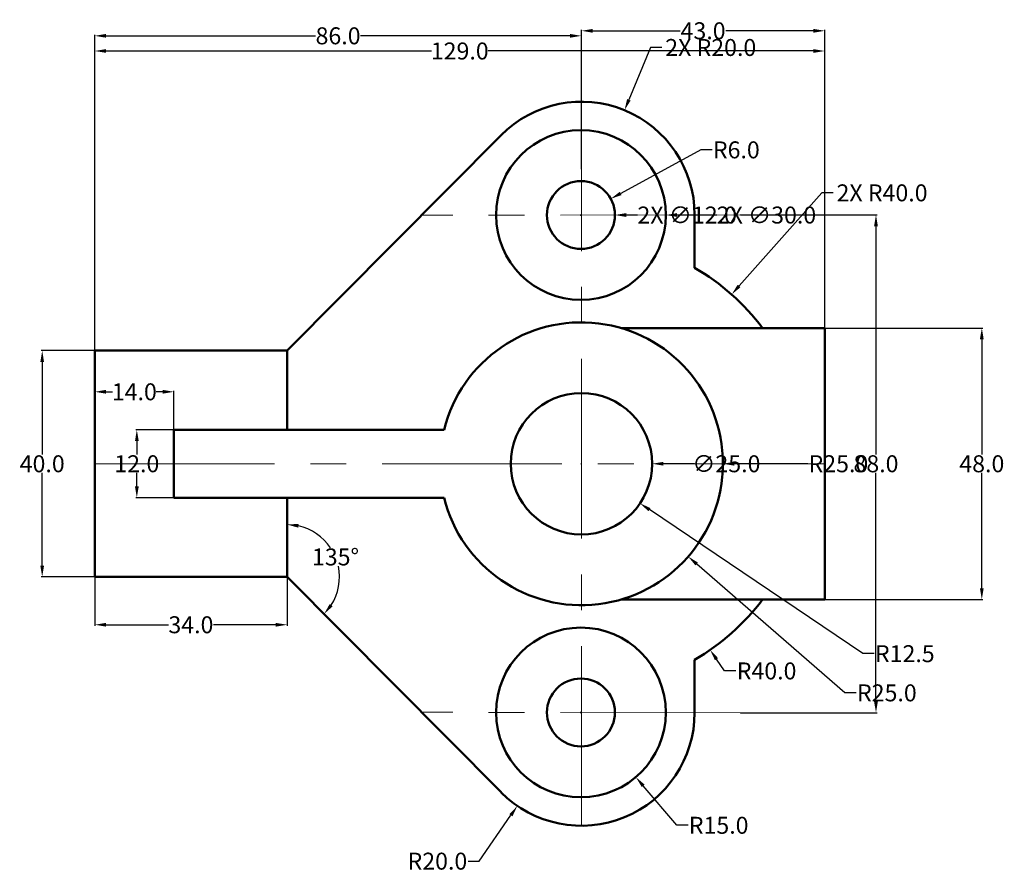
# Model space of a CAD drawing. Units: inches. Extents: x 158 to 332, y 82 to 233.
import ezdxf

# ---------------------------------------------------------------- set-up
doc = ezdxf.new("R2010")
doc.units = ezdxf.units.IN
doc.header["$MEASUREMENT"] = 0
doc.linetypes.add('CENTER', pattern=[50.8, 31.75, -6.35, 6.35, -6.35])
for name, color, linetype, lineweight in [('M-CNTR', 4, 'CENTER', 18), ('M-CONS', 8, 'Continuous', 13), ('M-DIMS', 2, 'Continuous', 25), ('M-OUTL', 7, 'Continuous', 50)]:
    doc.layers.add(name, color=color, linetype=linetype, lineweight=lineweight)
doc.styles.get("Standard").update_dxf_attribs({"font": 'arial.ttf'})
doc.dimstyles.get("Standard").update_dxf_attribs({"dimtxt": 3, "dimasz": 2, "dimexe": 0.18, "dimexo": 0.0625, "dimgap": 0.09, "dimtad": 0, "dimtih": 1, "dimtoh": 1, "dimdec": 1, "dimzin": 0, "dimdsep": 46, "dimtxsty": 'Standard', "dimcen": 0.09, "dimadec": 0, "dimazin": 0, "dimtfac": 1, "dimtdec": 1, "dimtofl": 0, "dimtmove": 0, "dimatfit": 3, "dimfxl": 1, "dimtolj": 1, "dimtzin": 0, "dimarcsym": 0})

# ---------------------------------------------------------------- blocks, each defined once
blk = doc.blocks.new('*D1')
at = {"layer": 'Defpoints', "color": 0, "transparency": 16777216}
for p in [(178.74, 160.59), (185.3, 160.59), (185.3, 148.59)]:
    blk.add_point(p, dxfattribs=at)
at = {"layer": 'M-DIMS', "color": 0, "lineweight": -2, "transparency": 16777216}
for p, q in [((185.24, 160.59), (178.56, 160.59)), ((178.74, 158.59), (178.74, 156.22)), ((178.74, 150.59), (178.74, 152.97)), ((185.24, 148.59), (178.56, 148.59))]:
    blk.add_line(p, q, dxfattribs=at)
at = {"layer": 'M-DIMS', "color": 0, "transparency": 16777216}
for points in [[(178.41, 158.59), (179.08, 158.59), (178.74, 160.59)], [(178.41, 150.59), (179.08, 150.59), (178.74, 148.59)]]:
    blk.add_solid(points, dxfattribs=at)
at = {"layer": 'M-DIMS', "color": 0, "transparency": 16777216, "insert": (178.74, 154.59), "char_height": 3, "attachment_point": 5}
blk.add_mtext('\\A1;12.0', dxfattribs=at)
blk = doc.blocks.new('*D2')
at = {"layer": 'Defpoints', "color": 0, "transparency": 16777216}
for p in [(171.3, 167.31), (185.3, 167.31), (185.3, 160.59)]:
    blk.add_point(p, dxfattribs=at)
at = {"layer": 'M-DIMS', "color": 0, "lineweight": -2, "transparency": 16777216}
for p, q in [((171.3, 167.38), (171.3, 167.49)), ((173.3, 167.31), (174.46, 167.31)), ((183.3, 167.31), (182.14, 167.31)), ((185.3, 160.66), (185.3, 167.49))]:
    blk.add_line(p, q, dxfattribs=at)
at = {"layer": 'M-DIMS', "color": 0, "transparency": 16777216}
for points in [[(173.3, 167.65), (173.3, 166.98), (171.3, 167.31)], [(183.3, 167.65), (183.3, 166.98), (185.3, 167.31)]]:
    blk.add_solid(points, dxfattribs=at)
at = {"layer": 'M-DIMS', "color": 0, "transparency": 16777216, "insert": (178.3, 167.31), "char_height": 3, "attachment_point": 5}
blk.add_mtext('\\A1;14.0', dxfattribs=at)
blk = doc.blocks.new('*D3')
at = {"layer": 'Defpoints', "color": 0, "transparency": 16777216}
for p in [(171.3, 134.59), (205.3, 134.59), (205.3, 126.13)]:
    blk.add_point(p, dxfattribs=at)
at = {"layer": 'M-DIMS', "color": 0, "lineweight": -2, "transparency": 16777216}
for p, q in [((171.3, 134.53), (171.3, 125.95)), ((205.3, 134.53), (205.3, 125.95)), ((173.3, 126.13), (184.32, 126.13)), ((203.3, 126.13), (192.28, 126.13))]:
    blk.add_line(p, q, dxfattribs=at)
at = {"layer": 'M-DIMS', "color": 0, "transparency": 16777216}
for points in [[(173.3, 126.46), (173.3, 125.8), (171.3, 126.13)], [(203.3, 126.46), (203.3, 125.8), (205.3, 126.13)]]:
    blk.add_solid(points, dxfattribs=at)
at = {"layer": 'M-DIMS', "color": 0, "transparency": 16777216, "insert": (188.3, 126.13), "char_height": 3, "attachment_point": 5}
blk.add_mtext('\\A1;34.0', dxfattribs=at)
blk = doc.blocks.new('*D4')
at = {"layer": 'Defpoints', "color": 0, "transparency": 16777216}
for p in [(162.02, 174.59), (171.3, 174.59), (171.3, 134.59)]:
    blk.add_point(p, dxfattribs=at)
at = {"layer": 'M-DIMS', "color": 0, "lineweight": -2, "transparency": 16777216}
for p, q in [((171.24, 174.59), (161.84, 174.59)), ((162.02, 172.59), (162.02, 156.22)), ((162.02, 136.59), (162.02, 152.97)), ((171.24, 134.59), (161.84, 134.59))]:
    blk.add_line(p, q, dxfattribs=at)
at = {"layer": 'M-DIMS', "color": 0, "transparency": 16777216}
for points in [[(161.69, 172.59), (162.35, 172.59), (162.02, 174.59)], [(161.69, 136.59), (162.35, 136.59), (162.02, 134.59)]]:
    blk.add_solid(points, dxfattribs=at)
at = {"layer": 'M-DIMS', "color": 0, "transparency": 16777216, "insert": (162.02, 154.59), "char_height": 3, "attachment_point": 5}
blk.add_mtext('\\A1;40.0', dxfattribs=at)
blk = doc.blocks.new('*D5')
at = {"layer": 'Defpoints', "color": 0, "transparency": 16777216}
for p in [(205.3, 148.59), (205.3, 134.59), (205.3, 134.59), (214.55, 134.57), (243.1, 96.51)]:
    blk.add_point(p, dxfattribs=at)
at = {"layer": 'M-DIMS', "color": 0, "lineweight": -2, "transparency": 16777216}
for start, end in [(33.8017, 77.592), (327.1935, 11.8638)]:
    blk.add_arc((205.3, 134.59), 9.25, start, end, dxfattribs=at)
at = {"layer": 'M-DIMS', "color": 0, "transparency": 16777216}
for points in [[(207.25, 143.3), (207.32, 143.96), (205.3, 143.85)], [(213.33, 129.37), (212.82, 129.79), (211.82, 128.03)]]:
    blk.add_solid(points, dxfattribs=at)
at = {"layer": 'M-DIMS', "color": 0, "transparency": 16777216, "insert": (213.85, 138.12), "char_height": 3, "attachment_point": 5}
blk.add_mtext('\\A1;135°', dxfattribs=at)
blk = doc.blocks.new('*D6')
at = {"layer": 'Defpoints', "color": 0, "transparency": 16777216}
for p in [(257.3, 110.59), (245.98, 94.11)]:
    blk.add_point(p, dxfattribs=at)
at = {"layer": 'M-DIMS', "color": 0, "lineweight": -2, "transparency": 16777216}
for p, q in [((257.21, 110.59), (257.39, 110.59)), ((257.3, 110.5), (257.3, 110.68)), ((239.26, 84.34), (244.84, 92.46)), ((237.26, 84.34), (239.26, 84.34))]:
    blk.add_line(p, q, dxfattribs=at)
at = {"layer": 'M-DIMS', "color": 0, "transparency": 16777216}
blk.add_solid([(244.57, 92.65), (245.12, 92.27), (245.98, 94.11)], dxfattribs=at)
at = {"layer": 'M-DIMS', "color": 0, "transparency": 16777216, "insert": (231.85, 84.34), "char_height": 3, "attachment_point": 5}
blk.add_mtext('\\A1;R20.0', dxfattribs=at)
blk = doc.blocks.new('*D7')
at = {"layer": 'Defpoints', "color": 0, "transparency": 16777216}
for p in [(257.21, 110.63), (266.92, 99.19)]:
    blk.add_point(p, dxfattribs=at)
at = {"layer": 'M-DIMS', "color": 0, "lineweight": -2, "transparency": 16777216}
for p, q in [((257.12, 110.63), (257.3, 110.63)), ((257.21, 110.54), (257.21, 110.72)), ((274.14, 90.68), (268.21, 97.67)), ((276.14, 90.68), (274.14, 90.68))]:
    blk.add_line(p, q, dxfattribs=at)
at = {"layer": 'M-DIMS', "color": 0, "transparency": 16777216}
blk.add_solid([(268.46, 97.88), (267.96, 97.45), (266.92, 99.19)], dxfattribs=at)
at = {"layer": 'M-DIMS', "color": 0, "transparency": 16777216, "insert": (281.55, 90.68), "char_height": 3, "attachment_point": 5}
blk.add_mtext('\\A1;R15.0', dxfattribs=at)
blk = doc.blocks.new('*D8')
at = {"layer": 'Defpoints', "color": 0, "transparency": 16777216}
for p in [(257.3, 154.59), (280.04, 121.69)]:
    blk.add_point(p, dxfattribs=at)
at = {"layer": 'M-DIMS', "color": 0, "lineweight": -2, "transparency": 16777216}
for p, q in [((257.21, 154.59), (257.39, 154.59)), ((257.3, 154.5), (257.3, 154.68)), ((282.61, 117.97), (281.17, 120.04)), ((284.61, 117.97), (282.61, 117.97))]:
    blk.add_line(p, q, dxfattribs=at)
at = {"layer": 'M-DIMS', "color": 0, "transparency": 16777216}
blk.add_solid([(281.45, 120.23), (280.9, 119.85), (280.04, 121.69)], dxfattribs=at)
at = {"layer": 'M-DIMS', "color": 0, "transparency": 16777216, "insert": (290.02, 117.97), "char_height": 3, "attachment_point": 5}
blk.add_mtext('\\A1;R40.0', dxfattribs=at)
blk = doc.blocks.new('*D9')
at = {"layer": 'Defpoints', "color": 0, "transparency": 16777216}
for p in [(257.3, 154.59), (276.16, 138.19)]:
    blk.add_point(p, dxfattribs=at)
at = {"layer": 'M-DIMS', "color": 0, "lineweight": -2, "transparency": 16777216}
for p, q in [((257.21, 154.59), (257.39, 154.59)), ((257.3, 154.5), (257.3, 154.68)), ((303.85, 114.09), (277.67, 136.87)), ((305.85, 114.09), (303.85, 114.09))]:
    blk.add_line(p, q, dxfattribs=at)
at = {"layer": 'M-DIMS', "color": 0, "transparency": 16777216}
blk.add_solid([(277.89, 137.12), (277.45, 136.62), (276.16, 138.19)], dxfattribs=at)
at = {"layer": 'M-DIMS', "color": 0, "transparency": 16777216, "insert": (311.27, 114.09), "char_height": 3, "attachment_point": 5}
blk.add_mtext('\\A1;R25.0', dxfattribs=at)
blk = doc.blocks.new('*D10')
at = {"layer": 'Defpoints', "color": 0, "transparency": 16777216}
for p in [(257.3, 154.59), (267.66, 147.6)]:
    blk.add_point(p, dxfattribs=at)
at = {"layer": 'M-DIMS', "color": 0, "lineweight": -2, "transparency": 16777216}
for p, q in [((257.21, 154.59), (257.39, 154.59)), ((257.3, 154.5), (257.3, 154.68)), ((307, 121.02), (269.31, 146.48)), ((309, 121.02), (307, 121.02))]:
    blk.add_line(p, q, dxfattribs=at)
at = {"layer": 'M-DIMS', "color": 0, "transparency": 16777216}
blk.add_solid([(269.5, 146.75), (269.13, 146.2), (267.66, 147.6)], dxfattribs=at)
at = {"layer": 'M-DIMS', "color": 0, "transparency": 16777216, "insert": (314.44, 121.02), "char_height": 3, "attachment_point": 5}
blk.add_mtext('\\A1;R12.5', dxfattribs=at)
blk = doc.blocks.new('*D11')
at = {"layer": 'Defpoints', "color": 0, "transparency": 16777216}
for p in [(300.3, 178.59), (300.3, 130.59), (328.05, 130.59)]:
    blk.add_point(p, dxfattribs=at)
at = {"layer": 'M-DIMS', "color": 0, "lineweight": -2, "transparency": 16777216}
for p, q in [((300.36, 178.59), (328.23, 178.59)), ((328.05, 176.59), (328.05, 156.22)), ((328.05, 132.59), (328.05, 152.97)), ((300.36, 130.59), (328.23, 130.59))]:
    blk.add_line(p, q, dxfattribs=at)
at = {"layer": 'M-DIMS', "color": 0, "transparency": 16777216}
for points in [[(327.71, 176.59), (328.38, 176.59), (328.05, 178.59)], [(327.71, 132.59), (328.38, 132.59), (328.05, 130.59)]]:
    blk.add_solid(points, dxfattribs=at)
at = {"layer": 'M-DIMS', "color": 0, "transparency": 16777216, "insert": (328.05, 154.59), "char_height": 3, "attachment_point": 5}
blk.add_mtext('\\A1;48.0', dxfattribs=at)
blk = doc.blocks.new('*D12')
at = {"layer": 'Defpoints', "color": 0, "transparency": 16777216}
for p in [(262.48, 201.43), (257.21, 198.56)]:
    blk.add_point(p, dxfattribs=at)
at = {"layer": 'M-DIMS', "color": 0, "lineweight": -2, "transparency": 16777216}
for p, q in [((278.42, 210.08), (264.24, 202.38)), ((280.42, 210.08), (278.42, 210.08)), ((257.12, 198.56), (257.3, 198.56)), ((257.21, 198.47), (257.21, 198.65))]:
    blk.add_line(p, q, dxfattribs=at)
at = {"layer": 'M-DIMS', "color": 0, "transparency": 16777216}
blk.add_solid([(264.08, 202.67), (264.4, 202.09), (262.48, 201.43)], dxfattribs=at)
at = {"layer": 'M-DIMS', "color": 0, "transparency": 16777216, "insert": (284.67, 210.08), "char_height": 3, "attachment_point": 5}
blk.add_mtext('\\A1;R6.0', dxfattribs=at)
blk = doc.blocks.new('*D13')
at = {"layer": 'Defpoints', "color": 0, "transparency": 16777216}
for p in [(257.3, 230.24), (257.3, 206.62), (171.3, 174.59)]:
    blk.add_point(p, dxfattribs=at)
at = {"layer": 'M-DIMS', "color": 0, "lineweight": -2, "transparency": 16777216}
for p, q in [((171.3, 174.66), (171.3, 230.42)), ((173.3, 230.24), (210.31, 230.24)), ((255.3, 230.24), (218.28, 230.24)), ((257.3, 206.69), (257.3, 230.42))]:
    blk.add_line(p, q, dxfattribs=at)
at = {"layer": 'M-DIMS', "color": 0, "transparency": 16777216}
for points in [[(173.3, 230.57), (173.3, 229.91), (171.3, 230.24)], [(255.3, 230.57), (255.3, 229.91), (257.3, 230.24)]]:
    blk.add_solid(points, dxfattribs=at)
at = {"layer": 'M-DIMS', "color": 0, "transparency": 16777216, "insert": (214.3, 230.24), "char_height": 3, "attachment_point": 5}
blk.add_mtext('\\A1;86.0', dxfattribs=at)
blk = doc.blocks.new('*D14')
at = {"layer": 'Defpoints', "color": 0, "transparency": 16777216}
for p in [(300.3, 231.13), (257.3, 223.28), (300.3, 178.59)]:
    blk.add_point(p, dxfattribs=at)
at = {"layer": 'M-DIMS', "color": 0, "lineweight": -2, "transparency": 16777216}
for p, q in [((257.3, 223.34), (257.3, 231.31)), ((259.3, 231.13), (274.76, 231.13)), ((298.3, 231.13), (282.84, 231.13)), ((300.3, 178.66), (300.3, 231.31))]:
    blk.add_line(p, q, dxfattribs=at)
at = {"layer": 'M-DIMS', "color": 0, "transparency": 16777216}
for points in [[(259.3, 231.46), (259.3, 230.79), (257.3, 231.13)], [(298.3, 231.46), (298.3, 230.79), (300.3, 231.13)]]:
    blk.add_solid(points, dxfattribs=at)
at = {"layer": 'M-DIMS', "color": 0, "transparency": 16777216, "insert": (278.8, 231.13), "char_height": 3, "attachment_point": 5}
blk.add_mtext('\\A1;43.0', dxfattribs=at)
blk = doc.blocks.new('CLEVIS-EAR-BORE')
for radius in [15, 6]:
    blk.add_circle((0, 0), radius)
blk = doc.blocks.new('*D16')
at = {"layer": 'Defpoints', "color": 0, "transparency": 16777216}
for p in [(285.36, 198.59), (309.35, 198.59), (285.36, 110.59)]:
    blk.add_point(p, dxfattribs=at)
at = {"layer": 'M-DIMS', "color": 0, "lineweight": -2, "transparency": 16777216}
for p, q in [((285.43, 198.59), (309.53, 198.59)), ((309.35, 196.59), (309.35, 156.22)), ((309.35, 112.59), (309.35, 152.97)), ((285.43, 110.59), (309.53, 110.59))]:
    blk.add_line(p, q, dxfattribs=at)
at = {"layer": 'M-DIMS', "color": 0, "transparency": 16777216}
for points in [[(309.01, 196.59), (309.68, 196.59), (309.35, 198.59)], [(309.01, 112.59), (309.68, 112.59), (309.35, 110.59)]]:
    blk.add_solid(points, dxfattribs=at)
at = {"layer": 'M-DIMS', "color": 0, "transparency": 16777216, "insert": (309.35, 154.59), "char_height": 3, "attachment_point": 5}
blk.add_mtext('\\A1;88.0', dxfattribs=at)
blk = doc.blocks.new('*D17')
at = {"layer": 'Defpoints', "color": 0, "transparency": 16777216}
for p in [(300.3, 227.56), (300.3, 178.59), (171.3, 174.59)]:
    blk.add_point(p, dxfattribs=at)
at = {"layer": 'M-DIMS', "color": 0, "lineweight": -2, "transparency": 16777216}
for p, q in [((171.3, 174.66), (171.3, 227.74)), ((173.3, 227.56), (230.79, 227.56)), ((298.3, 227.56), (240.8, 227.56)), ((300.3, 178.66), (300.3, 227.74))]:
    blk.add_line(p, q, dxfattribs=at)
at = {"layer": 'M-DIMS', "color": 0, "transparency": 16777216}
for points in [[(173.3, 227.89), (173.3, 227.23), (171.3, 227.56)], [(298.3, 227.89), (298.3, 227.23), (300.3, 227.56)]]:
    blk.add_solid(points, dxfattribs=at)
at = {"layer": 'M-DIMS', "color": 0, "transparency": 16777216, "insert": (235.8, 227.56), "char_height": 3, "attachment_point": 5}
blk.add_mtext('\\A1;129.0', dxfattribs=at)
blk = doc.blocks.new('*D18')
at = {"layer": 'Defpoints', "color": 0, "transparency": 16777216}
for p in [(251.21, 198.56), (263.21, 198.56)]:
    blk.add_point(p, dxfattribs=at)
at = {"layer": 'M-DIMS', "color": 0, "lineweight": -2, "transparency": 16777216}
for p, q in [((257.12, 198.56), (257.3, 198.56)), ((257.21, 198.47), (257.21, 198.65)), ((267.21, 198.56), (265.21, 198.56))]:
    blk.add_line(p, q, dxfattribs=at)
at = {"layer": 'M-DIMS', "color": 0, "transparency": 16777216}
blk.add_solid([(265.21, 198.9), (265.21, 198.23), (263.21, 198.56)], dxfattribs=at)
at = {"layer": 'M-DIMS', "color": 0, "transparency": 16777216, "insert": (275.99, 198.56), "char_height": 3, "attachment_point": 5}
blk.add_mtext('\\A1;2X ∅12.0', dxfattribs=at)
blk = doc.blocks.new('*D19')
at = {"layer": 'Defpoints', "color": 0, "transparency": 16777216}
for p in [(242.21, 198.56), (272.21, 198.56)]:
    blk.add_point(p, dxfattribs=at)
at = {"layer": 'M-DIMS', "color": 0, "lineweight": -2, "transparency": 16777216}
for p, q in [((257.12, 198.56), (257.3, 198.56)), ((257.21, 198.47), (257.21, 198.65)), ((281.21, 198.56), (274.21, 198.56))]:
    blk.add_line(p, q, dxfattribs=at)
at = {"layer": 'M-DIMS', "color": 0, "transparency": 16777216}
blk.add_solid([(274.21, 198.9), (274.21, 198.23), (272.21, 198.56)], dxfattribs=at)
at = {"layer": 'M-DIMS', "color": 0, "transparency": 16777216, "insert": (289.99, 198.56), "char_height": 3, "attachment_point": 5}
blk.add_mtext('\\A1;2X ∅30.0', dxfattribs=at)
blk = doc.blocks.new('*D20')
at = {"layer": 'Defpoints', "color": 0, "transparency": 16777216}
for p in [(264.92, 217.09), (257.3, 198.59)]:
    blk.add_point(p, dxfattribs=at)
at = {"layer": 'M-DIMS', "color": 0, "lineweight": -2, "transparency": 16777216}
for p, q in [((269.49, 228.18), (265.68, 218.94)), ((271.49, 228.18), (269.49, 228.18)), ((257.21, 198.59), (257.39, 198.59)), ((257.3, 198.5), (257.3, 198.68))]:
    blk.add_line(p, q, dxfattribs=at)
at = {"layer": 'M-DIMS', "color": 0, "transparency": 16777216}
blk.add_solid([(265.37, 219.06), (265.99, 218.81), (264.92, 217.09)], dxfattribs=at)
at = {"layer": 'M-DIMS', "color": 0, "transparency": 16777216, "insert": (280.15, 228.18), "char_height": 3, "attachment_point": 5}
blk.add_mtext('\\A1;2X R20.0', dxfattribs=at)
blk = doc.blocks.new('*D21')
at = {"layer": 'Defpoints', "color": 0, "transparency": 16777216}
for p in [(283.84, 184.52), (257.3, 154.59)]:
    blk.add_point(p, dxfattribs=at)
at = {"layer": 'M-DIMS', "color": 0, "lineweight": -2, "transparency": 16777216}
for p, q in [((299.76, 202.48), (285.16, 186.02)), ((301.76, 202.48), (299.76, 202.48)), ((257.21, 154.59), (257.39, 154.59)), ((257.3, 154.5), (257.3, 154.68))]:
    blk.add_line(p, q, dxfattribs=at)
at = {"layer": 'M-DIMS', "color": 0, "transparency": 16777216}
blk.add_solid([(284.91, 186.24), (285.41, 185.8), (283.84, 184.52)], dxfattribs=at)
at = {"layer": 'M-DIMS', "color": 0, "transparency": 16777216, "insert": (310.42, 202.48), "char_height": 3, "attachment_point": 5}
blk.add_mtext('\\A1;2X R40.0', dxfattribs=at)
blk = doc.blocks.new('*D22')
at = {"layer": 'Defpoints', "color": 0, "transparency": 16777216}
for p in [(257.3, 154.59), (282.3, 154.59)]:
    blk.add_point(p, dxfattribs=at)
at = {"layer": 'M-DIMS', "color": 0, "lineweight": -2, "transparency": 16777216}
for p, q in [((257.21, 154.59), (257.39, 154.59)), ((257.3, 154.5), (257.3, 154.68)), ((297.3, 154.59), (284.3, 154.59))]:
    blk.add_line(p, q, dxfattribs=at)
at = {"layer": 'M-DIMS', "color": 0, "transparency": 16777216}
blk.add_solid([(284.3, 154.93), (284.3, 154.26), (282.3, 154.59)], dxfattribs=at)
at = {"layer": 'M-DIMS', "color": 0, "transparency": 16777216, "insert": (302.71, 154.59), "char_height": 3, "attachment_point": 5}
blk.add_mtext('\\A1;R25.0', dxfattribs=at)
blk = doc.blocks.new('*D23')
at = {"layer": 'Defpoints', "color": 0, "transparency": 16777216}
for p in [(244.8, 154.59), (269.8, 154.59)]:
    blk.add_point(p, dxfattribs=at)
at = {"layer": 'M-DIMS', "color": 0, "lineweight": -2, "transparency": 16777216}
for p, q in [((257.21, 154.59), (257.39, 154.59)), ((257.3, 154.5), (257.3, 154.68)), ((277.3, 154.59), (271.8, 154.59))]:
    blk.add_line(p, q, dxfattribs=at)
at = {"layer": 'M-DIMS', "color": 0, "transparency": 16777216}
blk.add_solid([(271.8, 154.93), (271.8, 154.26), (269.8, 154.59)], dxfattribs=at)
at = {"layer": 'M-DIMS', "color": 0, "transparency": 16777216, "insert": (282.91, 154.59), "char_height": 3, "attachment_point": 5}
blk.add_mtext('\\A1;∅25.0', dxfattribs=at)

msp = doc.modelspace()

# ---------------------------------------------------------------- linework, layer by layer
at = {"layer": 'M-CNTR'}
for p, q in [((257.3, 90.59), (257.3, 206.62)), ((285.36, 198.59), (229.06, 198.53)), ((171.3, 154.59), (300.3, 154.59)), ((285.36, 110.59), (229.06, 110.66))]:
    msp.add_line(p, q, dxfattribs=at)
at = {"layer": 'M-CONS'}
msp.add_line((257.3, 114.59), (257.3, 110.59), dxfattribs=at)
at = {"layer": 'M-OUTL'}
for p, q in [((205.3, 174.59), (243.1, 212.68)), ((277.3, 198.59), (277.3, 189.24)), ((300.3, 178.59), (264.3, 178.59)), ((300.3, 154.59), (300.3, 178.59)), ((171.3, 134.59), (171.3, 174.59)), ((171.3, 174.59), (205.3, 174.59)), ((205.3, 174.59), (205.3, 160.59)), ((185.3, 148.59), (185.3, 160.59)), ((185.3, 160.59), (233.03, 160.59)), ((300.3, 154.59), (300.3, 130.59)), ((185.3, 148.59), (233.03, 148.59)), ((205.3, 148.59), (205.3, 134.59)), ((171.3, 134.59), (205.3, 134.59)), ((205.3, 134.59), (243.1, 96.51)), ((300.3, 130.59), (264.3, 130.59)), ((277.3, 110.59), (277.3, 119.95))]:
    msp.add_line(p, q, dxfattribs=at)
msp.add_circle((257.3, 154.59), 12.5, dxfattribs=at)
for centre, radius, start, end in [((257.3, 198.59), 20, 0, 135.2145), ((257.3, 154.59), 40, 36.8699, 60), ((257.3, 154.59), 25, 193.8865, 166.1135), ((257.3, 154.59), 40, 300, 323.1301), ((257.3, 110.59), 20, 224.7855, 0)]:
    msp.add_arc(centre, radius, start, end, dxfattribs=at)

# ---------------------------------------------------------------- block references
for p in [(257.21, 198.56), (257.21, 110.63)]:
    msp.add_blockref('CLEVIS-EAR-BORE', p, dxfattribs=at)

# ---------------------------------------------------------------- dimensions: what is measured, and where the dimension line sits
at = {"layer": 'M-DIMS'}
for base, p1, p2, picture, middle in [((257.3, 230.24), (171.3, 174.59), (257.3, 206.62), '*D13', (214.3, 230.24)), ((300.3, 231.13), (257.3, 223.28), (300.3, 178.59), '*D14', (278.8, 231.13))]:
    dim = msp.add_linear_dim(base=base, p1=p1, p2=p2, dimstyle='Standard', override={"dimclrd": 0, "dimclre": 0, "dimclrt": 0}, dxfattribs=at)
    dim.commit()
    dim.dimension.update_dxf_attribs({"geometry": picture, "text_midpoint": middle, "dimtype": 160})
for center, mpoint, picture, middle in [((257.3, 198.59), (264.92, 217.09), '*D20', (280.15, 228.18)), ((257.3, 154.59), (283.84, 184.52), '*D21', (310.42, 202.48))]:
    dim = msp.add_radius_dim(center=center, mpoint=mpoint, text='2X <>', dimstyle='Standard', override={"dimdec": 1, "dimlfac": 1, "dimrnd": 0, "dimzin": 0, "dimdsep": 46, "dimlunit": 2}, dxfattribs=at)
    dim.commit()
    dim.dimension.update_dxf_attribs({"geometry": picture, "text_midpoint": middle, "dimtype": 164})
for base, p1, p2, override, picture, middle in [((300.3, 227.56), (171.3, 174.59), (300.3, 178.59), {"dimdec": 1, "dimlfac": 1, "dimrnd": 0, "dimzin": 0, "dimdsep": 46, "dimlunit": 2}, '*D17', (235.8, 227.56)), ((205.3, 126.13), (171.3, 134.59), (205.3, 134.59), {"dimclrd": 0, "dimclre": 0, "dimclrt": 0}, '*D3', (188.3, 126.13))]:
    dim = msp.add_linear_dim(base=base, p1=p1, p2=p2, dimstyle='Standard', override=override, dxfattribs=at)
    dim.commit()
    dim.dimension.update_dxf_attribs({"geometry": picture, "text_midpoint": middle})
for center, mpoint, override, picture, middle in [((257.21, 198.56), (262.48, 201.43), {"dimclrd": 0, "dimclre": 0, "dimclrt": 0}, '*D12', (284.67, 210.08)), ((257.3, 154.59), (282.3, 154.59), {"dimdec": 1, "dimlfac": 1, "dimrnd": 0, "dimzin": 0, "dimdsep": 46, "dimlunit": 2}, '*D22', (297.3, 154.6)), ((257.3, 154.59), (280.04, 121.69), {"dimclrd": 0, "dimclre": 0, "dimclrt": 0}, '*D8', (290.02, 117.97)), ((257.3, 154.59), (276.16, 138.19), {"dimclrd": 0, "dimclre": 0, "dimclrt": 0}, '*D9', (311.27, 114.09)), ((257.3, 154.59), (267.66, 147.6), {"dimclrd": 0, "dimclre": 0, "dimclrt": 0}, '*D10', (314.44, 121.02)), ((257.3, 110.59), (245.98, 94.11), {"dimclrd": 0, "dimclre": 0, "dimclrt": 0}, '*D6', (231.85, 84.34)), ((257.21, 110.63), (266.92, 99.19), {"dimclrd": 0, "dimclre": 0, "dimclrt": 0}, '*D7', (281.55, 90.68))]:
    dim = msp.add_radius_dim(center=center, mpoint=mpoint, dimstyle='Standard', override=override, dxfattribs=at)
    dim.commit()
    dim.dimension.update_dxf_attribs({"geometry": picture, "text_midpoint": middle, "dimtype": 164})
for p1, p2, picture, middle in [((242.21, 198.56), (272.21, 198.56), '*D19', (281.21, 198.56)), ((251.21, 198.56), (263.21, 198.56), '*D18', (267.21, 198.56))]:
    dim = msp.add_diameter_dim_2p(p1=p1, p2=p2, text='2X <>', dimstyle='Standard', override={"dimdec": 1, "dimlfac": 1, "dimrnd": 0, "dimzin": 0, "dimdsep": 46, "dimlunit": 2}, dxfattribs=at)
    dim.commit()
    dim.dimension.update_dxf_attribs({"geometry": picture, "text_midpoint": middle, "dimtype": 163})
for base, p1, p2, angle, override, picture, middle in [((309.35, 198.59), (285.36, 110.59), (285.36, 198.59), 90, {"dimdec": 1, "dimlfac": 1, "dimrnd": 0, "dimzin": 0, "dimdsep": 46, "dimlunit": 2}, '*D16', (309.35, 154.59)), ((328.05, 130.59), (300.3, 178.59), (300.3, 130.59), 270, {"dimclrd": 0, "dimclre": 0, "dimclrt": 0}, '*D11', (328.05, 154.59)), ((162.02, 174.59), (171.3, 134.59), (171.3, 174.59), 90, {"dimclrd": 0, "dimclre": 0, "dimclrt": 0}, '*D4', (162.02, 154.59)), ((185.3, 167.31), (171.3, 167.31), (185.3, 160.59), 180, {"dimclrd": 0, "dimclre": 0, "dimclrt": 0}, '*D2', (178.3, 167.31)), ((178.74, 160.59), (185.3, 148.59), (185.3, 160.59), 90, {"dimclrd": 0, "dimclre": 0, "dimclrt": 0}, '*D1', (178.74, 154.59))]:
    dim = msp.add_linear_dim(base=base, p1=p1, p2=p2, angle=angle, dimstyle='Standard', override=override, dxfattribs=at)
    dim.commit()
    dim.dimension.update_dxf_attribs({"geometry": picture, "text_midpoint": middle})
dim = msp.add_diameter_dim_2p(p1=(244.8, 154.59), p2=(269.8, 154.59), dimstyle='Standard', override={"dimdec": 1, "dimlfac": 1, "dimrnd": 0, "dimzin": 0, "dimdsep": 46, "dimlunit": 2}, dxfattribs=at)
dim.commit()
dim.dimension.update_dxf_attribs({"geometry": '*D23', "text_midpoint": (277.3, 154.6), "dimtype": 163})
dim = msp.add_angular_dim_2l(base=(214.55, 134.57), line1=((205.3, 134.59), (243.1, 96.51)), line2=((205.3, 148.59), (205.3, 134.59)), dimstyle='Standard', override={"dimclrd": 0, "dimclre": 0, "dimclrt": 0}, dxfattribs=at)
dim.commit()
dim.dimension.update_dxf_attribs({"geometry": '*D5', "text_midpoint": (213.85, 138.12)})

doc.saveas('drawing.dxf')
